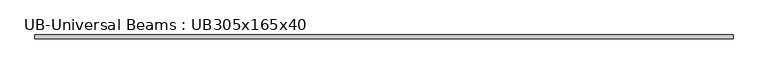
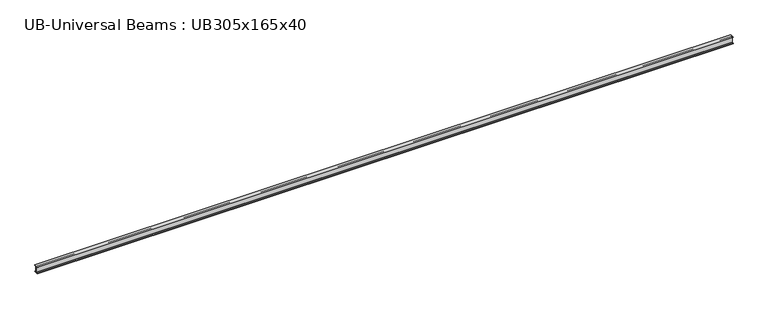
"""IFC4 building model written with IfcOpenShell, lengths in millimetres: beam geometry, UB-Universal Beams : UB305x165x40."""

from ifc_helpers import new_model, si_unit, point, frame, frame_2d, origin, place, context, project, spatial, polyline, circle_curve, trimmed, segment, composite_curve, outline, extrude, source, transform, mapped, element, save


def ub_universal_beams_ub305x165x40_c9eec61f(model_context):
    return source(origin(), model_context, "Body", "SweptSolid", [
        extrude(outline(composite_curve([segment(polyline([(82.5, -141.5), (82.5, -151.7), (-82.5, -151.7), (-82.5, -141.5), (-11.9, -141.5)]), True, "CONTINUOUS"), segment(trimmed(circle_curve(frame_2d((-11.9, -132.6)), 8.9), [point((-11.9, -141.5))], [point((-3.0, -132.6))], True, "CARTESIAN"), True, "CONTINUOUS"), segment(polyline([(-3.0, -132.6), (-3.0, 132.6)]), True, "CONTINUOUS"), segment(trimmed(circle_curve(frame_2d((-11.9, 132.6)), 8.9), [point((-3.0, 132.6))], [point((-11.9, 141.5))], True, "CARTESIAN"), True, "CONTINUOUS"), segment(polyline([(-11.9, 141.5), (-82.5, 141.5), (-82.5, 151.7), (82.5, 151.7), (82.5, 141.5), (11.9, 141.5)]), True, "CONTINUOUS"), segment(trimmed(circle_curve(frame_2d((11.9, 132.6)), 8.9), [point((11.9, 141.5))], [point((3.0, 132.6))], True, "CARTESIAN"), True, "CONTINUOUS"), segment(polyline([(3.0, 132.6), (3.0, -132.6)]), True, "CONTINUOUS"), segment(trimmed(circle_curve(frame_2d((11.9, -132.6)), 8.9), [point((3.0, -132.6))], [point((11.9, -141.5))], True, "CARTESIAN"), True, "CONTINUOUS"), segment(polyline([(11.9, -141.5), (82.5, -141.5)]), True, "CONTINUOUS")], self_intersect=False)), frame((-15240.0, 0.0, 0.0), z_axis=(1.0, 0.0, 0.0), x_axis=(0.0, 1.0, 0.0)), (0.0, 0.0, 1.0), 30480.0),
    ])


if __name__ == "__main__":
    model = new_model("IFC4")
    model_context = context("Model", 3, world=origin())
    ifc_project = project(units=[si_unit("LENGTHUNIT", "METRE", prefix="MILLI")], contexts=[model_context])
    site = spatial("IfcSite", under=ifc_project)
    building = spatial("IfcBuilding", under=site)
    placement = place(None, origin())
    ub_universal_beams_ub305x165x40_shape = ub_universal_beams_ub305x165x40_c9eec61f(model_context)
    element("IfcBeam", 1, ObjectType="UB-Universal Beams : UB305x165x40", at=placement, inside=building, context=model_context, shape_type="MappedRepresentation", body=[
        mapped(ub_universal_beams_ub305x165x40_shape, transform((0.0, 0.0, 0.0), x_axis=(1.0, 0.0, 0.0), y_axis=(0.0, 1.0, 0.0), z_axis=(0.0, 0.0, 1.0))),
    ])
    save(model, "model.ifc")

# Revit data of these elements
# Type "UB-Universal Beams : UB305x165x40"
#   Section Name Key = "UB305X165X40"
#   Width = 16.5 cm
#   Web Thickness = 0.6 cm
#   Web Fillet = 0.89 cm
#   Warping Constant = 164000.0 cm⁶
#   Torsional Moment of Inertia = 14.70 cm⁴
#   Section Area = 51.3 cm²
#   Plastic Modulus weak axis = 142.0 cm³
#   Plastic Modulus strong axis = 623.0 cm³
#   Nominal Weight = 40.2999 kgf/m
#   Moment of Inertia weak axis = 764.00 cm⁴
#   Moment of Inertia strong axis = 8503.00 cm⁴
#   Height = 30.34 cm
#   Flange Thickness = 1.02 cm
#   Elastic Modulus weak axis = 92.6 cm³
#   Elastic Modulus strong axis = 560.0 cm³
#   Centroid Vertical = 15.17 cm
#   Centroid Horizontal = 8.25 cm
#   Bolt Spacing = 9.0 cm
#   Length [instance default] = 1500 mm
#   Structural Material [instance default] = Metal - Steel 43-275
#   Type Comments = ""
#   Assembly Code = ""
# Element 1 (IfcBeam, "UB-Universal Beams : UB305x165x40")
#   Materials on its faces: "Metal - Steel 43-275"
# Materials
#   "Metal - Steel 43-275": class "Metal", colour RGB 247 247 247, transparency 0, Cost = 0
